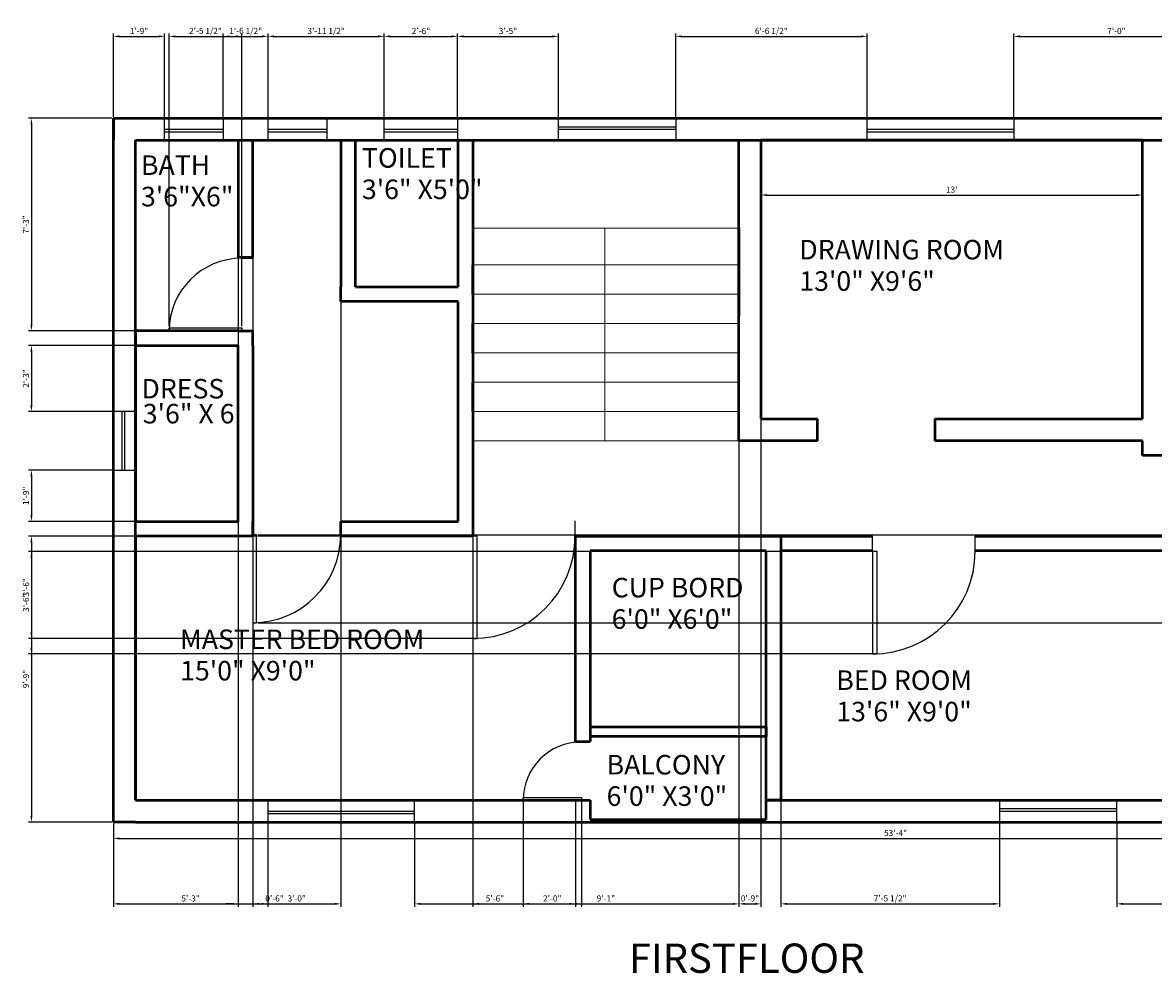
# Model space of a CAD drawing. Units: inches. Extents: x -5798 to 2718, y 1530 to 38999.
# Tile 1 of 4: x 2006 to 2468, y 1530 to 1919. Entities that reach past the tile are written whole.
import ezdxf

# ---------------------------------------------------------------- set-up
doc = ezdxf.new("R2010")
doc.units = ezdxf.units.IN
for name, color, linetype, lineweight in [('A-ANNO-DIMS', 2, 'Continuous', 18), ('A-ANNO-TEXT', 7, 'Continuous', 25), ('A-AREA-IDEN', 3, 'Continuous', 18), ('A-DOOR', 3, 'Continuous', 25), ('A-FLOR-STRS', 8, 'Continuous', 18), ('A-GLAZ', 4, 'Continuous', 25), ('A-WALL', 7, 'Continuous', 50)]:
    doc.layers.add(name, color=color, linetype=linetype, lineweight=lineweight)
doc.styles.get("Standard").update_dxf_attribs({"font": 'arial.ttf'})
doc.dimstyles.new('Copy of ISO-25', dxfattribs={"dimtxt": 2.5, "dimasz": 2.5, "dimexe": 1.25, "dimexo": 0.625, "dimtad": 1, "dimdec": 1, "dimlunit": 4, "dimtxsty": 'Standard', "dimcen": 2.5, "dimadec": 0, "dimazin": 0, "dimtfac": 1, "dimtdec": 1, "dimtmove": 0, "dimatfit": 3, "dimfxl": 1, "dimarcsym": 0})

# ---------------------------------------------------------------- blocks, each defined once
blk = doc.blocks.new('*U2')
for p, q in [((0, 0), (0, -6)), ((40, 0), (40, -6))]:
    blk.add_line(p, q)
blk.add_lwpolyline([(0, 0), (0, 40), (1.75, 40), (1.75, 0)], close=True)
blk.add_arc((0, 0), 40, 0, 90)
blk = doc.blocks.new('*U3')
for p, q in [((0, 0), (0, 6)), ((40, 0), (40, 6))]:
    blk.add_line(p, q)
blk.add_lwpolyline([(0, 0), (0, -40), (1.75, -40), (1.75, 0)], close=True)
blk.add_arc((0, 0), 40, 270, 0)
blk = doc.blocks.new('*D11')
at = {"layer": 'A-ANNO-DIMS', "color": 0, "lineweight": -2, "transparency": 16777216}
for p, q in [((2307.89, 1870.41), (2307.89, 1847.36)), ((2463.89, 1870.41), (2463.89, 1847.36)), ((2310.39, 1848.61), (2461.39, 1848.61))]:
    blk.add_line(p, q, dxfattribs=at)
at = {"layer": 'A-ANNO-DIMS', "color": 0, "transparency": 16777216}
for points in [[(2310.39, 1849.03), (2310.39, 1848.19), (2307.89, 1848.61)], [(2461.39, 1849.03), (2461.39, 1848.19), (2463.89, 1848.61)]]:
    blk.add_solid(points, dxfattribs=at)
at = {"layer": 'Defpoints', "color": 0, "transparency": 16777216}
for p in [(2307.89, 1871.03), (2463.89, 1871.03), (2463.89, 1848.61)]:
    blk.add_point(p, dxfattribs=at)
at = {"layer": 'A-ANNO-DIMS', "color": 0, "transparency": 16777216, "insert": (2385.89, 1850.51), "char_height": 2.5, "attachment_point": 5}
blk.add_mtext("13'", dxfattribs=at)
blk = doc.blocks.new('*D16')
at = {"layer": 'A-ANNO-DIMS', "color": 0, "lineweight": -2, "transparency": 16777216}
for p, q in [((2042.98, 1591.41), (2042.98, 1584.06)), ((2682.89, 1591.41), (2682.89, 1584.06)), ((2045.48, 1585.31), (2680.39, 1585.31))]:
    blk.add_line(p, q, dxfattribs=at)
at = {"layer": 'A-ANNO-DIMS', "color": 0, "transparency": 16777216}
for points in [[(2045.48, 1585.73), (2045.48, 1584.89), (2042.98, 1585.31)], [(2680.39, 1585.73), (2680.39, 1584.89), (2682.89, 1585.31)]]:
    blk.add_solid(points, dxfattribs=at)
at = {"layer": 'Defpoints', "color": 0, "transparency": 16777216}
for p in [(2042.98, 1592.03), (2682.89, 1592.03), (2682.89, 1585.31)]:
    blk.add_point(p, dxfattribs=at)
at = {"layer": 'A-ANNO-DIMS', "color": 0, "transparency": 16777216, "insert": (2362.93, 1587.21), "char_height": 2.5, "attachment_point": 5}
blk.add_mtext('53\'-4"', dxfattribs=at)
blk = doc.blocks.new('WIN-24')
for p, q in [((0, 0), (0, 9)), ((0, 9), (24, 9)), ((24, 9), (24, 0)), ((0, 4.5), (24, 4.5)), ((0, 3.5), (24, 3.5))]:
    blk.add_line(p, q)
blk = doc.blocks.new('WIN-48')
for p, q in [((0, 0), (0, 9)), ((0, 9), (48, 9)), ((0, 5.5), (48, 5.5)), ((48, 9), (48, 0)), ((0, 4.5), (48, 4.5))]:
    blk.add_line(p, q)
blk = doc.blocks.new('WIN-60')
for p, q in [((0, 0), (0, 9)), ((0, 9), (60, 9)), ((60, 9), (60, 0)), ((0, 4.5), (60, 4.5)), ((0, 3.5), (60, 3.5))]:
    blk.add_line(p, q)
blk = doc.blocks.new('WIN-48-B')
for p, q in [((0, 9), (0, 0)), ((0, 5.5), (48, 5.5)), ((48, 0), (48, 9)), ((0, 4.5), (48, 4.5)), ((0, 0), (48, 0))]:
    blk.add_line(p, q)
blk = doc.blocks.new('*D65')
at = {"layer": 'A-ANNO-DIMS', "color": 0, "lineweight": -2, "transparency": 16777216}
for p, q in [((2042.98, 1880.66), (2042.98, 1914.78)), ((2045.48, 1913.53), (2061.46, 1913.53)), ((2063.96, 1880.66), (2063.96, 1914.78))]:
    blk.add_line(p, q, dxfattribs=at)
at = {"layer": 'A-ANNO-DIMS', "color": 0, "transparency": 16777216}
for points in [[(2045.48, 1913.95), (2045.48, 1913.11), (2042.98, 1913.53)], [(2061.46, 1913.95), (2061.46, 1913.11), (2063.96, 1913.53)]]:
    blk.add_solid(points, dxfattribs=at)
at = {"layer": 'Defpoints', "color": 0, "transparency": 16777216}
for p in [(2063.96, 1913.53), (2042.98, 1880.03), (2063.96, 1880.03)]:
    blk.add_point(p, dxfattribs=at)
at = {"layer": 'A-ANNO-DIMS', "color": 0, "transparency": 16777216, "insert": (2053.47, 1915.43), "char_height": 2.5, "attachment_point": 5}
blk.add_mtext('1\'-9"', dxfattribs=at)
blk = doc.blocks.new('*D66')
at = {"layer": 'A-ANNO-DIMS', "color": 0, "lineweight": -2, "transparency": 16777216}
for p, q in [((2087.96, 1880.66), (2087.96, 1914.78)), ((2090.46, 1913.53), (2103.75, 1913.53)), ((2106.25, 1880.66), (2106.25, 1914.78))]:
    blk.add_line(p, q, dxfattribs=at)
at = {"layer": 'A-ANNO-DIMS', "color": 0, "transparency": 16777216}
for points in [[(2090.46, 1913.95), (2090.46, 1913.11), (2087.96, 1913.53)], [(2103.75, 1913.95), (2103.75, 1913.11), (2106.25, 1913.53)]]:
    blk.add_solid(points, dxfattribs=at)
at = {"layer": 'Defpoints', "color": 0, "transparency": 16777216}
for p in [(2106.25, 1913.53), (2087.96, 1880.03), (2106.25, 1880.03)]:
    blk.add_point(p, dxfattribs=at)
at = {"layer": 'A-ANNO-DIMS', "color": 0, "transparency": 16777216, "insert": (2097.1, 1915.45), "char_height": 2.5, "attachment_point": 5}
blk.add_mtext('1\'-6 1/2"', dxfattribs=at)
blk = doc.blocks.new('*D67')
at = {"layer": 'A-ANNO-DIMS', "color": 0, "lineweight": -2, "transparency": 16777216}
for p, q in [((2106.25, 1880.66), (2106.25, 1914.78)), ((2108.75, 1913.53), (2151.29, 1913.53)), ((2153.79, 1880.66), (2153.79, 1914.78))]:
    blk.add_line(p, q, dxfattribs=at)
at = {"layer": 'A-ANNO-DIMS', "color": 0, "transparency": 16777216}
for points in [[(2108.75, 1913.95), (2108.75, 1913.11), (2106.25, 1913.53)], [(2151.29, 1913.95), (2151.29, 1913.11), (2153.79, 1913.53)]]:
    blk.add_solid(points, dxfattribs=at)
at = {"layer": 'Defpoints', "color": 0, "transparency": 16777216}
for p in [(2153.79, 1913.53), (2106.25, 1880.03), (2153.79, 1880.03)]:
    blk.add_point(p, dxfattribs=at)
at = {"layer": 'A-ANNO-DIMS', "color": 0, "transparency": 16777216, "insert": (2130.02, 1915.45), "char_height": 2.5, "attachment_point": 5}
blk.add_mtext('3\'-11 1/2"', dxfattribs=at)
blk = doc.blocks.new('*D68')
at = {"layer": 'A-ANNO-DIMS', "color": 0, "lineweight": -2, "transparency": 16777216}
for p, q in [((2153.79, 1880.66), (2153.79, 1914.78)), ((2156.29, 1913.53), (2181.29, 1913.53)), ((2183.79, 1880.66), (2183.79, 1914.78))]:
    blk.add_line(p, q, dxfattribs=at)
at = {"layer": 'A-ANNO-DIMS', "color": 0, "transparency": 16777216}
for points in [[(2156.29, 1913.95), (2156.29, 1913.11), (2153.79, 1913.53)], [(2181.29, 1913.95), (2181.29, 1913.11), (2183.79, 1913.53)]]:
    blk.add_solid(points, dxfattribs=at)
at = {"layer": 'Defpoints', "color": 0, "transparency": 16777216}
for p in [(2183.79, 1913.53), (2153.79, 1880.03), (2183.79, 1880.03)]:
    blk.add_point(p, dxfattribs=at)
at = {"layer": 'A-ANNO-DIMS', "color": 0, "transparency": 16777216, "insert": (2168.79, 1915.43), "char_height": 2.5, "attachment_point": 5}
blk.add_mtext('2\'-6"', dxfattribs=at)
blk = doc.blocks.new('*D69')
at = {"layer": 'A-ANNO-DIMS', "color": 0, "lineweight": -2, "transparency": 16777216}
for p, q in [((2183.79, 1880.66), (2183.79, 1914.78)), ((2186.29, 1913.53), (2222.5, 1913.53)), ((2225, 1880.66), (2225, 1914.78))]:
    blk.add_line(p, q, dxfattribs=at)
at = {"layer": 'A-ANNO-DIMS', "color": 0, "transparency": 16777216}
for points in [[(2186.29, 1913.95), (2186.29, 1913.11), (2183.79, 1913.53)], [(2222.5, 1913.95), (2222.5, 1913.11), (2225, 1913.53)]]:
    blk.add_solid(points, dxfattribs=at)
at = {"layer": 'Defpoints', "color": 0, "transparency": 16777216}
for p in [(2225, 1913.53), (2183.79, 1880.03), (2225, 1880.03)]:
    blk.add_point(p, dxfattribs=at)
at = {"layer": 'A-ANNO-DIMS', "color": 0, "transparency": 16777216, "insert": (2204.39, 1915.43), "char_height": 2.5, "attachment_point": 5}
blk.add_mtext('3\'-5"', dxfattribs=at)
blk = doc.blocks.new('*D70')
at = {"layer": 'A-ANNO-DIMS', "color": 0, "lineweight": -2, "transparency": 16777216}
for p, q in [((2273, 1880.66), (2273, 1914.78)), ((2275.5, 1913.53), (2348.77, 1913.53)), ((2351.27, 1880.66), (2351.27, 1914.78))]:
    blk.add_line(p, q, dxfattribs=at)
at = {"layer": 'A-ANNO-DIMS', "color": 0, "transparency": 16777216}
for points in [[(2275.5, 1913.95), (2275.5, 1913.11), (2273, 1913.53)], [(2348.77, 1913.95), (2348.77, 1913.11), (2351.27, 1913.53)]]:
    blk.add_solid(points, dxfattribs=at)
at = {"layer": 'Defpoints', "color": 0, "transparency": 16777216}
for p in [(2351.27, 1913.53), (2273, 1880.03), (2351.27, 1880.03)]:
    blk.add_point(p, dxfattribs=at)
at = {"layer": 'A-ANNO-DIMS', "color": 0, "transparency": 16777216, "insert": (2312.13, 1915.45), "char_height": 2.5, "attachment_point": 5}
blk.add_mtext('6\'-6 1/2"', dxfattribs=at)
blk = doc.blocks.new('*D71')
at = {"layer": 'A-ANNO-DIMS', "color": 0, "lineweight": -2, "transparency": 16777216}
for p, q in [((2411.27, 1880.66), (2411.27, 1914.78)), ((2413.77, 1913.53), (2492.74, 1913.53)), ((2495.24, 1880.66), (2495.24, 1914.78))]:
    blk.add_line(p, q, dxfattribs=at)
at = {"layer": 'A-ANNO-DIMS', "color": 0, "transparency": 16777216}
for points in [[(2413.77, 1913.95), (2413.77, 1913.11), (2411.27, 1913.53)], [(2492.74, 1913.95), (2492.74, 1913.11), (2495.24, 1913.53)]]:
    blk.add_solid(points, dxfattribs=at)
at = {"layer": 'Defpoints', "color": 0, "transparency": 16777216}
for p in [(2495.24, 1913.53), (2411.27, 1880.03), (2495.24, 1880.03)]:
    blk.add_point(p, dxfattribs=at)
at = {"layer": 'A-ANNO-DIMS', "color": 0, "transparency": 16777216, "insert": (2453.26, 1915.43), "char_height": 2.5, "attachment_point": 5}
blk.add_mtext('7\'-0"', dxfattribs=at)
blk = doc.blocks.new('*D74')
at = {"layer": 'A-ANNO-DIMS', "color": 0, "lineweight": -2, "transparency": 16777216}
for p, q in [((2099.98, 1870.41), (2099.98, 1557.28)), ((2135.98, 1870.41), (2135.98, 1557.28)), ((2102.48, 1558.53), (2133.48, 1558.53))]:
    blk.add_line(p, q, dxfattribs=at)
at = {"layer": 'A-ANNO-DIMS', "color": 0, "transparency": 16777216}
for points in [[(2102.48, 1558.95), (2102.48, 1558.11), (2099.98, 1558.53)], [(2133.48, 1558.95), (2133.48, 1558.11), (2135.98, 1558.53)]]:
    blk.add_solid(points, dxfattribs=at)
at = {"layer": 'Defpoints', "color": 0, "transparency": 16777216}
for p in [(2099.98, 1871.03), (2135.98, 1871.03), (2135.98, 1558.53)]:
    blk.add_point(p, dxfattribs=at)
at = {"layer": 'A-ANNO-DIMS', "color": 0, "transparency": 16777216, "insert": (2117.98, 1560.43), "char_height": 2.5, "attachment_point": 5}
blk.add_mtext('3\'-0"', dxfattribs=at)
blk = doc.blocks.new('*D75')
at = {"layer": 'A-ANNO-DIMS', "color": 0, "lineweight": -2, "transparency": 16777216}
for p, q in [((2093.98, 1870.41), (2093.98, 1557.28)), ((2099.98, 1870.41), (2099.98, 1557.28)), ((2091.48, 1558.53), (2088.98, 1558.53)), ((2093.98, 1558.53), (2099.98, 1558.53)), ((2102.48, 1558.53), (2112.87, 1558.53))]:
    blk.add_line(p, q, dxfattribs=at)
at = {"layer": 'A-ANNO-DIMS', "color": 0, "transparency": 16777216}
for points in [[(2091.48, 1558.95), (2091.48, 1558.11), (2093.98, 1558.53)], [(2102.48, 1558.95), (2102.48, 1558.11), (2099.98, 1558.53)]]:
    blk.add_solid(points, dxfattribs=at)
at = {"layer": 'Defpoints', "color": 0, "transparency": 16777216}
for p in [(2093.98, 1871.03), (2099.98, 1871.03), (2099.98, 1558.53)]:
    blk.add_point(p, dxfattribs=at)
at = {"layer": 'A-ANNO-DIMS', "color": 0, "transparency": 16777216, "insert": (2108.92, 1560.43), "char_height": 2.5, "attachment_point": 5}
blk.add_mtext('0\'-6"', dxfattribs=at)
blk = doc.blocks.new('*D76')
at = {"layer": 'A-ANNO-DIMS', "color": 0, "lineweight": -2, "transparency": 16777216}
for p, q in [((2189.98, 1870.41), (2189.98, 1557.28)), ((2298.89, 1870.41), (2298.89, 1557.28)), ((2192.48, 1558.53), (2296.39, 1558.53))]:
    blk.add_line(p, q, dxfattribs=at)
at = {"layer": 'A-ANNO-DIMS', "color": 0, "transparency": 16777216}
for points in [[(2192.48, 1558.95), (2192.48, 1558.11), (2189.98, 1558.53)], [(2296.39, 1558.95), (2296.39, 1558.11), (2298.89, 1558.53)]]:
    blk.add_solid(points, dxfattribs=at)
at = {"layer": 'Defpoints', "color": 0, "transparency": 16777216}
for p in [(2189.98, 1871.03), (2298.89, 1871.03), (2298.89, 1558.53)]:
    blk.add_point(p, dxfattribs=at)
at = {"layer": 'A-ANNO-DIMS', "color": 0, "transparency": 16777216, "insert": (2244.43, 1560.43), "char_height": 2.5, "attachment_point": 5}
blk.add_mtext('9\'-1"', dxfattribs=at)
blk = doc.blocks.new('*D77')
at = {"layer": 'A-ANNO-DIMS', "color": 0, "lineweight": -2, "transparency": 16777216}
for p, q in [((2298.89, 1870.41), (2298.89, 1557.28)), ((2307.89, 1870.41), (2307.89, 1557.28)), ((2301.39, 1558.53), (2305.39, 1558.53))]:
    blk.add_line(p, q, dxfattribs=at)
at = {"layer": 'A-ANNO-DIMS', "color": 0, "transparency": 16777216}
for points in [[(2301.39, 1558.95), (2301.39, 1558.11), (2298.89, 1558.53)], [(2305.39, 1558.95), (2305.39, 1558.11), (2307.89, 1558.53)]]:
    blk.add_solid(points, dxfattribs=at)
at = {"layer": 'Defpoints', "color": 0, "transparency": 16777216}
for p in [(2298.89, 1871.03), (2307.89, 1871.03), (2307.89, 1558.53)]:
    blk.add_point(p, dxfattribs=at)
at = {"layer": 'A-ANNO-DIMS', "color": 0, "transparency": 16777216, "insert": (2303.39, 1560.43), "char_height": 2.5, "attachment_point": 5}
blk.add_mtext('0\'-9"', dxfattribs=at)
blk = doc.blocks.new('*D80')
at = {"layer": 'A-ANNO-DIMS', "color": 0, "lineweight": -2, "transparency": 16777216}
for p, q in [((2042.35, 1880.03), (2008.23, 1880.03)), ((2009.48, 1877.53), (2009.48, 1795.53)), ((2051.35, 1793.03), (2008.23, 1793.03))]:
    blk.add_line(p, q, dxfattribs=at)
at = {"layer": 'A-ANNO-DIMS', "color": 0, "transparency": 16777216}
for points in [[(2009.06, 1877.53), (2009.89, 1877.53), (2009.48, 1880.03)], [(2009.06, 1795.53), (2009.89, 1795.53), (2009.48, 1793.03)]]:
    blk.add_solid(points, dxfattribs=at)
at = {"layer": 'Defpoints', "color": 0, "transparency": 16777216}
for p in [(2042.98, 1880.03), (2009.48, 1793.03), (2051.98, 1793.03)]:
    blk.add_point(p, dxfattribs=at)
at = {"layer": 'A-ANNO-DIMS', "color": 0, "transparency": 16777216, "insert": (2007.57, 1836.53), "char_height": 2.5, "attachment_point": 5, "rotation": 90}
blk.add_mtext('7\'-3"', dxfattribs=at)
blk = doc.blocks.new('*D81')
at = {"layer": 'A-ANNO-DIMS', "color": 0, "lineweight": -2, "transparency": 16777216}
for p, q in [((2051.35, 1787.03), (2008.23, 1787.03)), ((2009.48, 1784.53), (2009.48, 1762.53)), ((2042.35, 1760.03), (2008.23, 1760.03))]:
    blk.add_line(p, q, dxfattribs=at)
at = {"layer": 'A-ANNO-DIMS', "color": 0, "transparency": 16777216}
for points in [[(2009.06, 1784.53), (2009.89, 1784.53), (2009.48, 1787.03)], [(2009.06, 1762.53), (2009.89, 1762.53), (2009.48, 1760.03)]]:
    blk.add_solid(points, dxfattribs=at)
at = {"layer": 'Defpoints', "color": 0, "transparency": 16777216}
for p in [(2051.98, 1787.03), (2009.48, 1760.03), (2042.98, 1760.03)]:
    blk.add_point(p, dxfattribs=at)
at = {"layer": 'A-ANNO-DIMS', "color": 0, "transparency": 16777216, "insert": (2007.57, 1773.53), "char_height": 2.5, "attachment_point": 5, "rotation": 90}
blk.add_mtext('2\'-3"', dxfattribs=at)
blk = doc.blocks.new('*D82')
at = {"layer": 'A-ANNO-DIMS', "color": 0, "lineweight": -2, "transparency": 16777216}
for p, q in [((2042.35, 1736.03), (2008.23, 1736.03)), ((2009.48, 1733.53), (2009.48, 1717.53)), ((2051.35, 1715.03), (2008.23, 1715.03))]:
    blk.add_line(p, q, dxfattribs=at)
at = {"layer": 'A-ANNO-DIMS', "color": 0, "transparency": 16777216}
for points in [[(2009.06, 1733.53), (2009.89, 1733.53), (2009.48, 1736.03)], [(2009.06, 1717.53), (2009.89, 1717.53), (2009.48, 1715.03)]]:
    blk.add_solid(points, dxfattribs=at)
at = {"layer": 'Defpoints', "color": 0, "transparency": 16777216}
for p in [(2042.98, 1736.03), (2009.48, 1715.03), (2051.98, 1715.03)]:
    blk.add_point(p, dxfattribs=at)
at = {"layer": 'A-ANNO-DIMS', "color": 0, "transparency": 16777216, "insert": (2007.57, 1725.53), "char_height": 2.5, "attachment_point": 5, "rotation": 90}
blk.add_mtext('1\'-9"', dxfattribs=at)
blk = doc.blocks.new('*D83')
at = {"layer": 'A-ANNO-DIMS', "color": 0, "lineweight": -2, "transparency": 16777216}
for p, q in [((2051.35, 1709.03), (2008.23, 1709.03)), ((2009.48, 1706.53), (2009.48, 1594.53)), ((2042.35, 1592.03), (2008.23, 1592.03))]:
    blk.add_line(p, q, dxfattribs=at)
at = {"layer": 'A-ANNO-DIMS', "color": 0, "transparency": 16777216}
for points in [[(2009.06, 1706.53), (2009.89, 1706.53), (2009.48, 1709.03)], [(2009.06, 1594.53), (2009.89, 1594.53), (2009.48, 1592.03)]]:
    blk.add_solid(points, dxfattribs=at)
at = {"layer": 'Defpoints', "color": 0, "transparency": 16777216}
for p in [(2051.98, 1709.03), (2009.48, 1592.03), (2042.98, 1592.03)]:
    blk.add_point(p, dxfattribs=at)
at = {"layer": 'A-ANNO-DIMS', "color": 0, "transparency": 16777216, "insert": (2007.57, 1650.53), "char_height": 2.5, "attachment_point": 5, "rotation": 90}
blk.add_mtext('9\'-9"', dxfattribs=at)
blk = doc.blocks.new('*D87')
at = {"layer": 'A-ANNO-DIMS', "color": 0, "lineweight": -2, "transparency": 16777216}
for p, q in [((2042.98, 1591.41), (2042.98, 1557.28)), ((2106.16, 1591.41), (2106.16, 1557.28)), ((2045.48, 1558.53), (2103.66, 1558.53))]:
    blk.add_line(p, q, dxfattribs=at)
at = {"layer": 'A-ANNO-DIMS', "color": 0, "transparency": 16777216}
for points in [[(2045.48, 1558.95), (2045.48, 1558.11), (2042.98, 1558.53)], [(2103.66, 1558.95), (2103.66, 1558.11), (2106.16, 1558.53)]]:
    blk.add_solid(points, dxfattribs=at)
at = {"layer": 'Defpoints', "color": 0, "transparency": 16777216}
for p in [(2042.98, 1592.03), (2106.16, 1592.03), (2106.16, 1558.53)]:
    blk.add_point(p, dxfattribs=at)
at = {"layer": 'A-ANNO-DIMS', "color": 0, "transparency": 16777216, "insert": (2074.57, 1560.43), "char_height": 2.5, "attachment_point": 5}
blk.add_mtext('5\'-3"', dxfattribs=at)
blk = doc.blocks.new('*D88')
at = {"layer": 'A-ANNO-DIMS', "color": 0, "lineweight": -2, "transparency": 16777216}
for p, q in [((2231.98, 1600.41), (2231.98, 1557.28)), ((2166.16, 1591.41), (2166.16, 1557.28)), ((2168.66, 1558.53), (2229.48, 1558.53))]:
    blk.add_line(p, q, dxfattribs=at)
at = {"layer": 'A-ANNO-DIMS', "color": 0, "transparency": 16777216}
for points in [[(2168.66, 1558.95), (2168.66, 1558.11), (2166.16, 1558.53)], [(2229.48, 1558.95), (2229.48, 1558.11), (2231.98, 1558.53)]]:
    blk.add_solid(points, dxfattribs=at)
at = {"layer": 'Defpoints', "color": 0, "transparency": 16777216}
for p in [(2231.98, 1601.03), (2166.16, 1592.03), (2231.98, 1558.53)]:
    blk.add_point(p, dxfattribs=at)
at = {"layer": 'A-ANNO-DIMS', "color": 0, "transparency": 16777216, "insert": (2199.07, 1560.43), "char_height": 2.5, "attachment_point": 5}
blk.add_mtext('5\'-6"', dxfattribs=at)
blk = doc.blocks.new('*D89')
at = {"layer": 'A-ANNO-DIMS', "color": 0, "lineweight": -2, "transparency": 16777216}
for p, q in [((2315.98, 1600.41), (2315.98, 1557.28)), ((2405.45, 1591.41), (2405.45, 1557.28)), ((2318.48, 1558.53), (2402.95, 1558.53))]:
    blk.add_line(p, q, dxfattribs=at)
at = {"layer": 'A-ANNO-DIMS', "color": 0, "transparency": 16777216}
for points in [[(2318.48, 1558.95), (2318.48, 1558.11), (2315.98, 1558.53)], [(2402.95, 1558.95), (2402.95, 1558.11), (2405.45, 1558.53)]]:
    blk.add_solid(points, dxfattribs=at)
at = {"layer": 'Defpoints', "color": 0, "transparency": 16777216}
for p in [(2315.98, 1601.03), (2405.45, 1592.03), (2405.45, 1558.53)]:
    blk.add_point(p, dxfattribs=at)
at = {"layer": 'A-ANNO-DIMS', "color": 0, "transparency": 16777216, "insert": (2360.71, 1560.45), "char_height": 2.5, "attachment_point": 5}
blk.add_mtext('7\'-5 1/2"', dxfattribs=at)
blk = doc.blocks.new('*D90')
at = {"layer": 'A-ANNO-DIMS', "color": 0, "lineweight": -2, "transparency": 16777216}
for p, q in [((2511.89, 1600.41), (2511.89, 1557.28)), ((2453.45, 1591.41), (2453.45, 1557.28)), ((2455.95, 1558.53), (2509.39, 1558.53))]:
    blk.add_line(p, q, dxfattribs=at)
at = {"layer": 'A-ANNO-DIMS', "color": 0, "transparency": 16777216}
for points in [[(2455.95, 1558.95), (2455.95, 1558.11), (2453.45, 1558.53)], [(2509.39, 1558.95), (2509.39, 1558.11), (2511.89, 1558.53)]]:
    blk.add_solid(points, dxfattribs=at)
at = {"layer": 'Defpoints', "color": 0, "transparency": 16777216}
for p in [(2511.89, 1601.03), (2453.45, 1592.03), (2511.89, 1558.53)]:
    blk.add_point(p, dxfattribs=at)
at = {"layer": 'A-ANNO-DIMS', "color": 0, "transparency": 16777216, "insert": (2482.67, 1560.45), "char_height": 2.5, "attachment_point": 5}
blk.add_mtext('4\'-10 1/2"', dxfattribs=at)
blk = doc.blocks.new('*D93')
at = {"layer": 'A-ANNO-DIMS', "color": 0, "lineweight": -2, "transparency": 16777216}
for p, q in [((2065.81, 1794.96), (2065.81, 1914.78)), ((2068.31, 1913.53), (2093.02, 1913.53)), ((2095.52, 1794.96), (2095.52, 1914.78))]:
    blk.add_line(p, q, dxfattribs=at)
at = {"layer": 'A-ANNO-DIMS', "color": 0, "transparency": 16777216}
for points in [[(2068.31, 1913.95), (2068.31, 1913.11), (2065.81, 1913.53)], [(2093.02, 1913.95), (2093.02, 1913.11), (2095.52, 1913.53)]]:
    blk.add_solid(points, dxfattribs=at)
at = {"layer": 'Defpoints', "color": 0, "transparency": 16777216}
for p in [(2095.52, 1913.53), (2065.81, 1794.33), (2095.52, 1794.33)]:
    blk.add_point(p, dxfattribs=at)
at = {"layer": 'A-ANNO-DIMS', "color": 0, "transparency": 16777216, "insert": (2080.66, 1915.45), "char_height": 2.5, "attachment_point": 5}
blk.add_mtext('2\'-5 1/2"', dxfattribs=at)
blk = doc.blocks.new('*D94')
at = {"layer": 'A-ANNO-DIMS', "color": 0, "lineweight": -2, "transparency": 16777216}
for p, q in [((2102.18, 1709.6), (2717.64, 1709.6)), ((2716.39, 1707.1), (2716.39, 1676.07)), ((2102.18, 1673.57), (2717.64, 1673.57))]:
    blk.add_line(p, q, dxfattribs=at)
at = {"layer": 'A-ANNO-DIMS', "color": 0, "transparency": 16777216}
for points in [[(2715.98, 1707.1), (2716.81, 1707.1), (2716.39, 1709.6)], [(2715.98, 1676.07), (2716.81, 1676.07), (2716.39, 1673.57)]]:
    blk.add_solid(points, dxfattribs=at)
at = {"layer": 'Defpoints', "color": 0, "transparency": 16777216}
for p in [(2101.55, 1709.6), (2101.55, 1673.57), (2716.39, 1673.57)]:
    blk.add_point(p, dxfattribs=at)
at = {"layer": 'A-ANNO-DIMS', "color": 0, "transparency": 16777216, "insert": (2714.49, 1691.59), "char_height": 2.5, "attachment_point": 5, "rotation": 90}
blk.add_mtext('3\'-0"', dxfattribs=at)
blk = doc.blocks.new('*D95')
at = {"layer": 'A-ANNO-DIMS', "color": 0, "lineweight": -2, "transparency": 16777216}
for p, q in [((2191.18, 1709.03), (2008.23, 1709.03)), ((2009.48, 1706.53), (2009.48, 1669.62)), ((2191.18, 1667.12), (2008.23, 1667.12))]:
    blk.add_line(p, q, dxfattribs=at)
at = {"layer": 'A-ANNO-DIMS', "color": 0, "transparency": 16777216}
for points in [[(2009.06, 1706.53), (2009.89, 1706.53), (2009.48, 1709.03)], [(2009.06, 1669.62), (2009.89, 1669.62), (2009.48, 1667.12)]]:
    blk.add_solid(points, dxfattribs=at)
at = {"layer": 'Defpoints', "color": 0, "transparency": 16777216}
for p in [(2191.81, 1709.03), (2009.48, 1667.12), (2191.81, 1667.12)]:
    blk.add_point(p, dxfattribs=at)
at = {"layer": 'A-ANNO-DIMS', "color": 0, "transparency": 16777216, "insert": (2007.57, 1688.07), "char_height": 2.5, "attachment_point": 5, "rotation": 90}
blk.add_mtext('3\'-6"', dxfattribs=at)
blk = doc.blocks.new('*D96')
at = {"layer": 'A-ANNO-DIMS', "color": 0, "lineweight": -2, "transparency": 16777216}
for p, q in [((2210.61, 1601.45), (2210.61, 1557.28)), ((2234.41, 1601.45), (2234.41, 1557.28)), ((2213.11, 1558.53), (2231.91, 1558.53))]:
    blk.add_line(p, q, dxfattribs=at)
at = {"layer": 'A-ANNO-DIMS', "color": 0, "transparency": 16777216}
for points in [[(2213.11, 1558.95), (2213.11, 1558.11), (2210.61, 1558.53)], [(2231.91, 1558.95), (2231.91, 1558.11), (2234.41, 1558.53)]]:
    blk.add_solid(points, dxfattribs=at)
at = {"layer": 'Defpoints', "color": 0, "transparency": 16777216}
for p in [(2210.61, 1602.07), (2234.41, 1602.07), (2234.41, 1558.53)]:
    blk.add_point(p, dxfattribs=at)
at = {"layer": 'A-ANNO-DIMS', "color": 0, "transparency": 16777216, "insert": (2222.51, 1560.43), "char_height": 2.5, "attachment_point": 5}
blk.add_mtext('2\'-0"', dxfattribs=at)
blk = doc.blocks.new('*D97')
at = {"layer": 'A-ANNO-DIMS', "color": 0, "lineweight": -2, "transparency": 16777216}
for p, q in [((2354.78, 1702.74), (2008.23, 1702.74)), ((2009.48, 1700.24), (2009.48, 1663.33)), ((2354.78, 1660.83), (2008.23, 1660.83))]:
    blk.add_line(p, q, dxfattribs=at)
at = {"layer": 'A-ANNO-DIMS', "color": 0, "transparency": 16777216}
for points in [[(2009.06, 1700.24), (2009.89, 1700.24), (2009.48, 1702.74)], [(2009.06, 1663.33), (2009.89, 1663.33), (2009.48, 1660.83)]]:
    blk.add_solid(points, dxfattribs=at)
at = {"layer": 'Defpoints', "color": 0, "transparency": 16777216}
for p in [(2355.41, 1702.74), (2009.48, 1660.83), (2355.41, 1660.83)]:
    blk.add_point(p, dxfattribs=at)
at = {"layer": 'A-ANNO-DIMS', "color": 0, "transparency": 16777216, "insert": (2007.57, 1681.79), "char_height": 2.5, "attachment_point": 5, "rotation": 90}
blk.add_mtext('3\'-6"', dxfattribs=at)

msp = doc.modelspace()

# ---------------------------------------------------------------- linework, layer by layer
at = {"layer": 'A-FLOR-STRS'}
for p, q in [((2189.98, 1835.03), (2298.89, 1835.03)), ((2189.98, 1835.03), (2225.98, 1835.03)), ((2189.98, 1835.03), (2243.98, 1835.03)), ((2243.98, 1835.03), (2243.98, 1748.03)), ((2189.98, 1820.03), (2298.89, 1820.03)), ((2298.89, 1808.03), (2189.98, 1808.03)), ((2189.98, 1796.03), (2298.89, 1796.03)), ((2298.89, 1784.03), (2189.98, 1784.03)), ((2189.98, 1772.03), (2298.89, 1772.03)), ((2298.89, 1760.03), (2189.98, 1760.03)), ((2243.98, 1748.03), (2189.98, 1748.03)), ((2243.98, 1748.03), (2298.89, 1748.03))]:
    msp.add_line(p, q, dxfattribs=at)
at = {"layer": 'A-GLAZ'}
for p, q in [((2153.79, 1871.03), (2153.79, 1880.03)), ((2153.79, 1880.03), (2183.79, 1880.03)), ((2183.79, 1880.03), (2183.79, 1871.03)), ((2153.79, 1875.53), (2183.79, 1875.53)), ((2153.79, 1874.53), (2183.79, 1874.53)), ((2051.98, 1760.03), (2042.98, 1760.03)), ((2042.98, 1760.03), (2042.98, 1736.03)), ((2046.48, 1760.03), (2046.48, 1736.03)), ((2047.48, 1760.03), (2047.48, 1736.03)), ((2051.98, 1736.03), (2051.98, 1760.03)), ((2042.98, 1736.03), (2051.98, 1736.03)), ((2106.16, 1601.03), (2106.16, 1592.03)), ((2166.16, 1592.03), (2166.16, 1601.03)), ((2106.16, 1596.53), (2166.16, 1596.53)), ((2106.16, 1595.53), (2166.16, 1595.53)), ((2106.16, 1592.03), (2166.16, 1592.03))]:
    msp.add_line(p, q, dxfattribs=at)
at = {"layer": 'A-WALL'}
for p, q in [((2042.98, 1880.03), (2682.89, 1880.03)), ((2042.98, 1592.03), (2042.98, 1880.03)), ((2042.98, 1880.03), (2042.98, 1871.03)), ((2051.98, 1871.03), (2673.89, 1871.03)), ((2051.98, 1601.03), (2051.98, 1871.03)), ((2051.98, 1871.03), (2093.98, 1871.03)), ((2051.98, 1871.03), (2063.96, 1871.03)), ((2093.98, 1871.03), (2093.98, 1823.03)), ((2099.98, 1823.03), (2099.98, 1871.03)), ((2099.98, 1871.03), (2135.98, 1871.03)), ((2099.98, 1871.03), (2106.25, 1871.03)), ((2135.98, 1871.03), (2135.98, 1811.03)), ((2141.98, 1811.03), (2141.98, 1871.03)), ((2141.98, 1871.03), (2141.98, 1871.03)), ((2141.98, 1871.03), (2153.79, 1871.03)), ((2183.98, 1811.03), (2183.98, 1871.03)), ((2183.98, 1871.03), (2189.98, 1871.03)), ((2189.98, 1871.03), (2189.98, 1811.03)), ((2189.98, 1871.03), (2189.98, 1835.03)), ((2189.98, 1871.03), (2225, 1871.03)), ((2298.89, 1748.03), (2298.89, 1871.03)), ((2463.89, 1871.03), (2307.89, 1871.03)), ((2307.89, 1871.03), (2307.89, 1757.03)), ((2307.89, 1871.03), (2351.27, 1871.03)), ((2463.89, 1757.03), (2463.89, 1871.03)), ((2298.89, 1835.03), (2298.89, 1799.03)), ((2099.98, 1823.03), (2093.98, 1823.03)), ((2189.98, 1808.03), (2189.98, 1820.03)), ((2135.98, 1805.03), (2135.98, 1811.03)), ((2141.98, 1811.03), (2183.98, 1811.03)), ((2189.98, 1811.03), (2189.98, 1805.03)), ((2183.98, 1805.03), (2135.98, 1805.03)), ((2183.98, 1715.03), (2183.98, 1805.03)), ((2189.98, 1805.03), (2189.98, 1709.03)), ((2298.89, 1796.03), (2298.89, 1808.03)), ((2189.98, 1784.03), (2189.98, 1796.03)), ((2093.98, 1793.03), (2051.98, 1793.03)), ((2051.98, 1793.03), (2051.98, 1787.03)), ((2093.98, 1793.03), (2099.98, 1793.03)), ((2099.98, 1787.03), (2099.98, 1793.03)), ((2051.98, 1787.03), (2093.98, 1787.03)), ((2051.98, 1787.03), (2051.98, 1715.03)), ((2093.98, 1715.03), (2093.98, 1787.03)), ((2099.98, 1787.03), (2099.98, 1715.03)), ((2298.89, 1772.03), (2298.89, 1784.03)), ((2189.98, 1760.03), (2189.98, 1772.03)), ((2298.89, 1748.03), (2298.89, 1760.03)), ((2307.89, 1757.03), (2331.04, 1757.03)), ((2307.89, 1757.03), (2331.04, 1757.03)), ((2331.04, 1748.03), (2331.04, 1757.03)), ((2379.04, 1757.03), (2379.04, 1748.03)), ((2379.04, 1757.03), (2463.89, 1757.03)), ((2307.89, 1748.03), (2298.89, 1748.03)), ((2331.04, 1748.03), (2307.89, 1748.03)), ((2463.89, 1748.03), (2379.04, 1748.03)), ((2463.89, 1742.03), (2463.89, 1748.03)), ((2472.89, 1742.03), (2463.89, 1742.03)), ((2051.98, 1715.03), (2051.98, 1736.03)), ((2051.98, 1715.03), (2093.98, 1715.03)), ((2099.98, 1715.03), (2099.98, 1709.03)), ((2099.98, 1709.03), (2099.98, 1715.03)), ((2135.98, 1715.03), (2183.98, 1715.03)), ((2135.98, 1709.03), (2135.98, 1715.03)), ((2099.98, 1709.03), (2051.98, 1709.03)), ((2051.98, 1709.03), (2051.98, 1601.03)), ((2051.98, 1709.03), (2051.98, 1601.03)), ((2189.98, 1709.03), (2135.98, 1709.03)), ((2231.98, 1625.03), (2231.98, 1709.03)), ((2231.98, 1709.03), (2237.98, 1709.03)), ((2237.98, 1709.03), (2309.98, 1709.03)), ((2309.98, 1709.03), (2315.98, 1709.03)), ((2315.98, 1709.03), (2315.98, 1601.03)), ((2315.98, 1709.03), (2353.57, 1709.03)), ((2395.48, 1709.03), (2577.89, 1709.03)), ((2309.98, 1703.03), (2237.98, 1703.03)), ((2237.98, 1703.03), (2237.98, 1625.03)), ((2237.98, 1703.03), (2237.98, 1631.03)), ((2309.98, 1601.03), (2309.98, 1703.03)), ((2353.57, 1703.03), (2315.98, 1703.03)), ((2511.89, 1703.03), (2395.48, 1703.03)), ((2237.98, 1631.03), (2309.98, 1631.03)), ((2309.98, 1631.03), (2309.98, 1627.03)), ((2231.98, 1625.03), (2237.98, 1625.03)), ((2309.98, 1627.03), (2237.98, 1627.03)), ((2051.98, 1601.03), (2231.98, 1601.03)), ((2051.98, 1601.03), (2231.98, 1601.03)), ((2051.98, 1601.03), (2106.16, 1601.03)), ((2231.98, 1601.03), (2237.98, 1601.03)), ((2237.98, 1601.03), (2237.98, 1593.03)), ((2309.98, 1601.03), (2673.89, 1601.03)), ((2315.98, 1601.03), (2309.98, 1601.03)), ((2309.98, 1593.03), (2309.98, 1601.03)), ((2042.98, 1592.03), (2042.98, 1597.32)), ((2051.98, 1592.03), (2042.98, 1592.03)), ((2051.98, 1592.03), (2231.98, 1592.03)), ((2231.98, 1592.03), (2237.98, 1592.03)), ((2237.98, 1593.03), (2309.98, 1593.03)), ((2237.98, 1592.03), (2673.89, 1592.03))]:
    msp.add_line(p, q, dxfattribs=at)

# ---------------------------------------------------------------- block references
at = {"layer": 'A-DOOR', "rotation": 90}
for p, xscale, yscale, zscale in [((2095.52, 1793.03), 0.7427986004694425, 0.7427986004694425, 0.7427986004694425), ((2234.41, 1601.03), 0.5948199903653146, 0.5948199903653146, 0.5948199903653146)]:
    msp.add_blockref('*U2', p, dxfattribs=dict(at, xscale=xscale, yscale=yscale, zscale=zscale))
at = {"layer": 'A-DOOR'}
for p, xscale, yscale, zscale in [((2099.98, 1709.6), 0.9005998972476804, 0.9005998972476804, 0.9005998972476804), ((2189.98, 1709.03), 1.047776570873516, 1.047776570873516, 1.047776570873516), ((2353.57, 1702.74), 1.047776570873516, 1.047776570873516, 1.047776570873516)]:
    msp.add_blockref('*U3', p, dxfattribs=dict(at, xscale=xscale, yscale=yscale, zscale=zscale))
at = {"layer": 'A-GLAZ'}
for name, p in [('WIN-24', (2063.96, 1871.03)), ('WIN-24', (2106.25, 1871.03)), ('WIN-48', (2225, 1871.03)), ('WIN-60', (2351.27, 1871.03)), ('WIN-48-B', (2405.45, 1592.03))]:
    msp.add_blockref(name, p, dxfattribs=at)

# ---------------------------------------------------------------- texts
at = {"layer": 'A-ANNO-TEXT', "insert": (2253.82, 1542.29), "char_height": 12, "attachment_point": 1}
msp.add_mtext_dynamic_manual_height_columns(' FIRSTFLOOR                                     ', width=7.4566, gutter_width=60, heights=[0], dxfattribs=at)
at = {"layer": 'A-AREA-IDEN'}
for s, p in [('BATH', (2054.29, 1856.83)), ('TOILET', (2144.66, 1859.81)), ('3\'6" X5\'0"', (2144.66, 1846.96)), ('3\'6"X6"', (2054.29, 1843.98)), ('DRAWING ROOM', (2323.58, 1822.26)), ('13\'0" X9\'6"', (2323.58, 1809.41)), ('DRESS', (2054.49, 1765.35)), ('3\'6" X 6\'', (2055.02, 1755.14)), ('CUP BORD', (2246.83, 1683.95)), ('6\'0" X6\'0"', (2246.83, 1671.1)), ('MASTER BED ROOM', (2070.3, 1662.81)), ('15\'0" X9\'0"', (2070.3, 1649.96)), ('BED ROOM ', (2338.7, 1646.07)), ('13\'6" X9\'0"', (2338.7, 1633.22)), ('BALCONY', (2244.74, 1611.48)), ('6\'0" X3\'0"', (2244.74, 1598.63))]:
    msp.add_text(s, height=8, dxfattribs=at).set_placement(p)

# ---------------------------------------------------------------- dimensions: what is measured, and where the dimension line sits
at = {"layer": 'A-ANNO-DIMS'}
for base, p1, p2, override, picture, middle in [((2063.96, 1913.53), (2042.98, 1880.03), (2063.96, 1880.03), {"dimdec": 1, "dimlfac": 1, "dimrnd": 0, "dimzin": 1, "dimdsep": 46, "dimlunit": 4, "dimfrac": 2}, '*D65', (2053.47, 1915.43)), ((2095.52, 1913.53), (2065.81, 1794.33), (2095.52, 1794.33), {"dimdec": 1, "dimlfac": 1, "dimrnd": 0, "dimzin": 1, "dimdsep": 46, "dimlunit": 4, "dimfrac": 2}, '*D93', (2080.66, 1915.45)), ((2106.25, 1913.53), (2087.96, 1880.03), (2106.25, 1880.03), {"dimdec": 1, "dimlfac": 1, "dimrnd": 0, "dimzin": 1, "dimdsep": 46, "dimlunit": 4, "dimfrac": 2}, '*D66', (2097.1, 1915.45)), ((2153.79, 1913.53), (2106.25, 1880.03), (2153.79, 1880.03), {"dimdec": 1, "dimlfac": 1, "dimrnd": 0, "dimzin": 1, "dimdsep": 46, "dimlunit": 4, "dimfrac": 2}, '*D67', (2130.02, 1915.45)), ((2183.79, 1913.53), (2153.79, 1880.03), (2183.79, 1880.03), {"dimdec": 1, "dimlfac": 1, "dimrnd": 0, "dimzin": 1, "dimdsep": 46, "dimlunit": 4, "dimfrac": 2}, '*D68', (2168.79, 1915.43)), ((2225, 1913.53), (2183.79, 1880.03), (2225, 1880.03), {"dimdec": 1, "dimlfac": 1, "dimrnd": 0, "dimzin": 1, "dimdsep": 46, "dimlunit": 4, "dimfrac": 2}, '*D69', (2204.39, 1915.43)), ((2351.27, 1913.53), (2273, 1880.03), (2351.27, 1880.03), {"dimdec": 1, "dimlfac": 1, "dimrnd": 0, "dimzin": 1, "dimdsep": 46, "dimlunit": 4, "dimfrac": 2}, '*D70', (2312.13, 1915.45)), ((2495.24, 1913.53), (2411.27, 1880.03), (2495.24, 1880.03), {"dimdec": 1, "dimlfac": 1, "dimrnd": 0, "dimzin": 1, "dimdsep": 46, "dimlunit": 4, "dimfrac": 2}, '*D71', (2453.26, 1915.43)), ((2099.98, 1558.53), (2093.98, 1871.03), (2099.98, 1871.03), {"dimdec": 1, "dimlfac": 1, "dimrnd": 0, "dimzin": 1, "dimdsep": 46, "dimlunit": 4, "dimfrac": 2}, '*D75', (2108.92, 1560.43)), ((2135.98, 1558.53), (2099.98, 1871.03), (2135.98, 1871.03), {"dimdec": 1, "dimlfac": 1, "dimrnd": 0, "dimzin": 1, "dimdsep": 46, "dimlunit": 4, "dimfrac": 2}, '*D74', (2117.98, 1560.43)), ((2298.89, 1558.53), (2189.98, 1871.03), (2298.89, 1871.03), {"dimdec": 1, "dimlfac": 1, "dimrnd": 0, "dimzin": 1, "dimdsep": 46, "dimlunit": 4, "dimfrac": 2}, '*D76', (2244.43, 1560.43)), ((2307.89, 1558.53), (2298.89, 1871.03), (2307.89, 1871.03), {"dimdec": 1, "dimlfac": 1, "dimrnd": 0, "dimzin": 1, "dimdsep": 46, "dimlunit": 4, "dimfrac": 2}, '*D77', (2303.39, 1560.43)), ((2463.89, 1848.61), (2307.89, 1871.03), (2463.89, 1871.03), {"dimclrd": 0, "dimclre": 0, "dimclrt": 0}, '*D11', (2385.89, 1850.51)), ((2231.98, 1558.53), (2166.16, 1592.03), (2231.98, 1601.03), {"dimdec": 1, "dimlfac": 1, "dimrnd": 0, "dimzin": 1, "dimdsep": 46, "dimlunit": 4, "dimfrac": 2}, '*D88', (2199.07, 1560.43)), ((2234.41, 1558.53), (2210.61, 1602.07), (2234.41, 1602.07), {"dimdec": 1, "dimlfac": 1, "dimrnd": 0, "dimzin": 1, "dimdsep": 46, "dimlunit": 4, "dimfrac": 2}, '*D96', (2222.51, 1560.43)), ((2405.45, 1558.53), (2315.98, 1601.03), (2405.45, 1592.03), {"dimdec": 1, "dimlfac": 1, "dimrnd": 0, "dimzin": 1, "dimdsep": 46, "dimlunit": 4, "dimfrac": 2}, '*D89', (2360.71, 1560.45)), ((2511.89, 1558.53), (2453.45, 1592.03), (2511.89, 1601.03), {"dimdec": 1, "dimlfac": 1, "dimrnd": 0, "dimzin": 1, "dimdsep": 46, "dimlunit": 4, "dimfrac": 2}, '*D90', (2482.67, 1560.45)), ((2682.89, 1585.31), (2042.98, 1592.03), (2682.89, 1592.03), {"dimclrd": 0, "dimclre": 0, "dimclrt": 0}, '*D16', (2362.93, 1587.21)), ((2106.16, 1558.53), (2042.98, 1592.03), (2106.16, 1592.03), {"dimdec": 1, "dimlfac": 1, "dimrnd": 0, "dimzin": 1, "dimdsep": 46, "dimlunit": 4, "dimfrac": 2}, '*D87', (2074.57, 1560.43))]:
    dim = msp.add_linear_dim(base=base, p1=p1, p2=p2, dimstyle='Copy of ISO-25', override=override, dxfattribs=at)
    dim.commit()
    dim.dimension.update_dxf_attribs({"geometry": picture, "text_midpoint": middle})
for base, p1, p2, picture, middle in [((2009.48, 1793.03), (2042.98, 1880.03), (2051.98, 1793.03), '*D80', (2007.57, 1836.53)), ((2009.48, 1760.03), (2051.98, 1787.03), (2042.98, 1760.03), '*D81', (2007.57, 1773.53)), ((2009.48, 1715.03), (2042.98, 1736.03), (2051.98, 1715.03), '*D82', (2007.57, 1725.53)), ((2009.48, 1592.03), (2051.98, 1709.03), (2042.98, 1592.03), '*D83', (2007.57, 1650.53)), ((2009.48, 1667.12), (2191.81, 1709.03), (2191.81, 1667.12), '*D95', (2007.57, 1688.07)), ((2716.39, 1673.57), (2101.55, 1709.6), (2101.55, 1673.57), '*D94', (2714.49, 1691.59)), ((2009.48, 1660.83), (2355.41, 1702.74), (2355.41, 1660.83), '*D97', (2007.57, 1681.79))]:
    dim = msp.add_linear_dim(base=base, p1=p1, p2=p2, angle=90, dimstyle='Copy of ISO-25', override={"dimdec": 1, "dimlfac": 1, "dimrnd": 0, "dimzin": 1, "dimdsep": 46, "dimlunit": 4, "dimfrac": 2}, dxfattribs=at)
    dim.commit()
    dim.dimension.update_dxf_attribs({"geometry": picture, "text_midpoint": middle})

doc.saveas('drawing.dxf')
